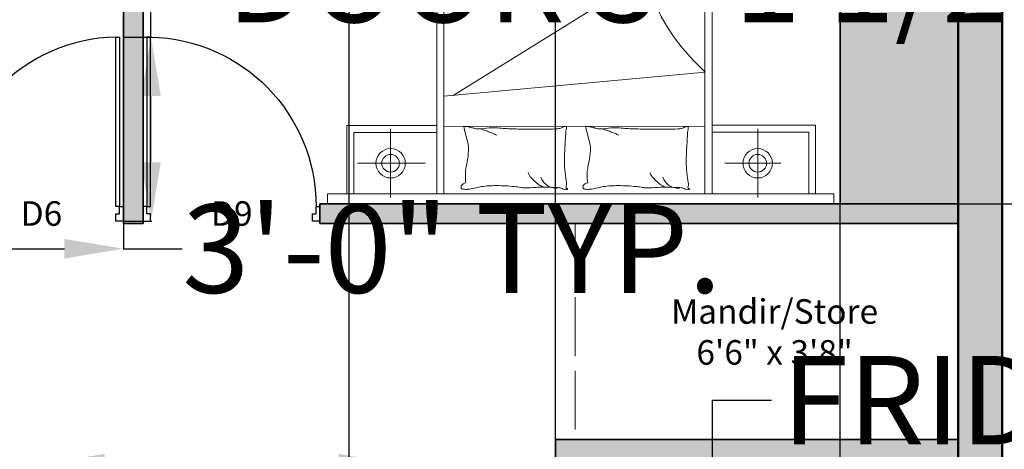
# Model space of a CAD drawing. Units: inches. Extents: x 2796 to 3603, y 978 to 1787.
# Tile 11 of 15: x 3224 to 3425, y 1458 to 1545. Entities that reach past the tile are written whole.
import ezdxf

# ---------------------------------------------------------------- set-up
doc = ezdxf.new("R2010")
doc.units = ezdxf.units.IN
doc.linetypes.add('ACAD_ISO02W100', pattern=[15, 12, -3])
for name, color, linetype, lineweight in [('A-ANNO-DIMS', 7, 'Continuous', 18), ('A-ANNO-TEXT', 7, 'Continuous', 18), ('A-AREA-IDEN', 7, 'Continuous', 18), ('A-DOOR', 6, 'Continuous', 25), ('A-FLOR-CASE', 2, 'Continuous', 25), ('A-FLOR-CASE-PATT', 2, 'Continuous', 13), ('A-FLOR-OVHD', 7, 'ACAD_ISO02W100', 18), ('A-WALL-EXTR-PATT', 1, 'Continuous', 13), ('A-WALL-INTR-PATT', 5, 'Continuous', 13), ('Furniture', 2, 'Continuous', 18), ('Inner Wall', 5, 'Continuous', 35), ('Outer Wall', 1, 'Continuous', 50)]:
    doc.layers.add(name, color=color, linetype=linetype, lineweight=lineweight)
doc.styles.get("Standard").update_dxf_attribs({"font": 'arial.ttf'})
doc.dimstyles.get("Standard").update_dxf_attribs({"dimtxt": 18, "dimasz": 12, "dimexe": 0.18, "dimexo": 0.0625, "dimgap": 0.09, "dimtad": 0, "dimtih": 1, "dimtoh": 1, "dimdec": 0, "dimzin": 0, "dimdsep": 46, "dimlunit": 3, "dimtxsty": 'Standard', "dimcen": 0.09, "dimadec": 0, "dimazin": 0, "dimtfac": 1, "dimtdec": 0, "dimtofl": 0, "dimtmove": 0, "dimatfit": 3, "dimfxl": 1, "dimtolj": 1, "dimtzin": 0, "dimarcsym": 0})

# ---------------------------------------------------------------- blocks, each defined once
blk = doc.blocks.new('A$C2B723114')
for p, q in [((0, 2.9047), (2.8274, 2.9047)), ((0, 2.8487), (0, 2.9047)), ((0.4243, 2.8697), (0.4243, 2.4855)), ((2.4742, 2.8697), (2.4742, 2.4855)), ((2.8274, 2.9047), (2.8274, 2.8487)), ((2.8274, 2.8487), (0, 2.8487)), ((0.1012, 2.4649), (0.1012, 2.849)), ((0.1396, 2.5033), (0.1396, 2.849)), ((0.6794, 0.7051), (0.6794, 2.8509)), ((0.7187, 0.7435), (0.7187, 2.8509)), ((2.1776, 2.8509), (2.1776, 0.7454)), ((2.216, 2.8509), (2.216, 0.707)), ((2.6798, 2.5052), (2.6798, 2.8509)), ((2.7182, 2.4668), (2.7182, 2.8509)), ((0.6087, 2.6776), (0.295, 2.6776)), ((2.6586, 2.6776), (2.2821, 2.6776)), ((1.3789, 2.4999), (1.3598, 2.5761)), ((2.0593, 2.4999), (2.0402, 2.5761)), ((0.6766, 2.5033), (0.1396, 2.5033)), ((1.3858, 2.4723), (1.3789, 2.4999)), ((2.0662, 2.4723), (2.0593, 2.4999)), ((2.2188, 2.5052), (2.6798, 2.5052)), ((0.6794, 2.4649), (0.1012, 2.4649)), ((0.7191, 2.47), (2.1778, 2.4719)), ((2.2188, 2.4668), (2.7182, 2.4668)), ((2.1771, 2.3036), (0.718, 2.1685)), ((1.0365, 1.6233), (2.1246, 2.2989)), ((2.2287, 1.6076), (2.2523, 1.5035)), ((0.5047, 1.5819), (0.5353, 1.4945)), ((0.6174, 1.5819), (0.6232, 1.4916)), ((0.6467, 1.5819), (0.6369, 1.5137)), ((0.6571, 1.4945), (0.6571, 1.5765)), ((2.2726, 1.593), (2.3061, 1.5007)), ((2.3067, 1.5881), (2.3373, 1.5007)), ((2.4194, 1.5881), (2.4251, 1.4979)), ((2.4487, 1.5881), (2.4389, 1.5199)), ((2.4591, 1.5007), (2.4591, 1.5828)), ((0.4269, 0.0884), (0.4269, 1.4945)), ((0.4269, 1.4945), (0.6794, 1.4945)), ((2.4685, 1.4964), (2.216, 1.5022)), ((2.4685, 1.4964), (2.4685, 0.0903)), ((0.3172, 1.3923), (0.4213, 1.3687)), ((2.4685, 1.4044), (2.5491, 1.3861)), ((0.3318, 1.3485), (0.4241, 1.3149)), ((2.4596, 1.3659), (2.552, 1.3324)), ((2.4645, 1.3318), (2.552, 1.3012)), ((0.3367, 1.3143), (0.4241, 1.2838)), ((2.4645, 1.2928), (2.5548, 1.2871)), ((2.4645, 1.2635), (2.5328, 1.2733)), ((2.4699, 1.2531), (2.552, 1.2163)), ((2.552, 1.2531), (2.4699, 1.2531)), ((2.5435, 1.2276), (2.4699, 1.2163)), ((2.4699, 1.2163), (2.5463, 1.1823)), ((0.3367, 1.2016), (0.427, 1.1959)), ((0.3367, 1.1724), (0.405, 1.1821)), ((0.4241, 1.162), (0.3421, 1.162)), ((0.3421, 1.162), (0.4241, 1.1252)), ((2.5491, 1.1654), (2.467, 1.1597)), ((2.5463, 1.1455), (2.467, 1.1342)), ((2.5491, 1.1342), (2.4699, 1.1201)), ((2.4699, 1.1201), (2.5491, 1.0946)), ((2.5463, 1.1172), (2.4727, 1.0918)), ((2.5491, 1.0946), (2.4699, 1.0635)), ((2.4699, 1.0635), (2.5491, 0.9842)), ((0.4157, 1.0206), (0.3421, 1.0093)), ((0.3421, 1.0093), (0.4185, 0.9754)), ((2.4642, 1.0267), (2.552, 0.9644)), ((0.4213, 0.9584), (0.3392, 0.9527)), ((0.4185, 0.9386), (0.3392, 0.9272)), ((2.4642, 0.9389), (2.4869, 0.9276)), ((2.467, 0.9559), (2.552, 0.9333)), ((2.4699, 0.9785), (2.552, 0.9531)), ((0.4213, 0.9272), (0.3421, 0.9131)), ((0.3421, 0.9131), (0.4213, 0.8876)), ((0.4213, 0.8876), (0.3421, 0.8565)), ((0.4185, 0.9103), (0.3449, 0.8848)), ((2.4642, 0.8908), (2.5152, 0.8483)), ((2.4869, 0.9276), (2.5265, 0.9163)), ((2.5265, 0.9163), (2.5491, 0.9163)), ((0.3421, 0.8565), (0.4213, 0.7772)), ((2.467, 0.8455), (2.5208, 0.8342)), ((2.5152, 0.8483), (2.5491, 0.837)), ((2.5208, 0.8342), (2.552, 0.8285)), ((2.552, 0.8285), (2.5293, 0.8087)), ((0.3364, 0.8197), (0.4241, 0.7574)), ((0.3421, 0.7716), (0.4241, 0.7461)), ((2.5491, 0.7606), (2.467, 0.7719)), ((2.4699, 0.8172), (2.4925, 0.7974)), ((2.5491, 0.8087), (2.4699, 0.8172)), ((2.4925, 0.7974), (2.535, 0.7889)), ((2.535, 0.7889), (2.552, 0.7861)), ((0.3392, 0.7489), (0.4241, 0.7263)), ((0.359, 0.7206), (0.3987, 0.7093)), ((2.1776, 0.7454), (0.7187, 0.7435)), ((2.4727, 0.7464), (2.467, 0.7408)), ((2.467, 0.7153), (2.5491, 0.7238)), ((2.552, 0.7464), (2.4727, 0.7464)), ((0.3421, 0.6601), (0.4213, 0.5808)), ((0.3987, 0.7093), (0.4213, 0.7093)), ((2.216, 0.707), (0.6794, 0.7051)), ((0.9938, 0.6115), (1.7555, 0.7064)), ((2.5491, 0.6842), (2.4642, 0.6615)), ((2.552, 0.7096), (2.467, 0.6842)), ((2.5491, 0.6672), (2.4755, 0.6587)), ((0.3364, 0.6233), (0.4241, 0.561)), ((2.4642, 0.6191), (2.4784, 0.6134)), ((2.4755, 0.6474), (2.5548, 0.6276)), ((2.4784, 0.6134), (2.5406, 0.6077)), ((2.5406, 0.6077), (2.552, 0.6134)), ((0.3392, 0.5525), (0.4241, 0.5299)), ((0.3421, 0.5752), (0.4241, 0.5497)), ((2.467, 0.5993), (2.4869, 0.5964)), ((2.467, 0.5313), (2.5491, 0.5596)), ((2.4869, 0.5964), (2.552, 0.5964)), ((0.359, 0.5242), (0.3987, 0.5129)), ((1.4523, 0.5021), (1.1305, 0.4537)), ((2.467, 0.5087), (2.5548, 0.5342)), ((2.5548, 0.5342), (2.4699, 0.4889)), ((0.3364, 0.4785), (0.3874, 0.436)), ((1.1305, 0.4537), (0.9938, 0.448)), ((0.4213, 0.415), (0.3364, 0.3923)), ((0.3392, 0.4332), (0.393, 0.4219)), ((0.4241, 0.2868), (0.3392, 0.415)), ((0.3421, 0.4049), (0.3647, 0.3851)), ((0.4213, 0.3964), (0.3421, 0.4049)), ((0.4213, 0.398), (0.3477, 0.3895)), ((0.3647, 0.3851), (0.4072, 0.3766)), ((0.3874, 0.436), (0.4213, 0.4247)), ((0.393, 0.4219), (0.4241, 0.4162)), ((0.4241, 0.4162), (0.4015, 0.3964)), ((2.467, 0.4133), (2.552, 0.4019)), ((2.467, 0.2879), (2.552, 0.4076)), ((0.4213, 0.3377), (0.3392, 0.3491)), ((0.4072, 0.3766), (0.4241, 0.3738)), ((0.3392, 0.2925), (0.4213, 0.3009)), ((0.4241, 0.3236), (0.3449, 0.3236)), ((2.4642, 0.3049), (2.5491, 0.2851)), ((2.467, 0.319), (2.5548, 0.3134)), ((0.3477, 0.2571), (0.427, 0.2373)), ((0.3506, 0.2231), (0.4128, 0.2175)), ((0.4128, 0.2175), (0.4241, 0.2231)), ((2.4699, 0.2491), (2.501, 0.2491)), ((2.501, 0.2491), (2.5491, 0.2547)), ((0.359, 0.2061), (0.4241, 0.2061)), ((2.467, 0.2179), (2.5605, 0.1981)), ((2.467, 0.1981), (2.5491, 0.1613)), ((2.467, 0.184), (2.4982, 0.1755)), ((2.4982, 0.1755), (2.5463, 0.1359)), ((0.3392, 0.1042), (0.4213, 0.1325)), ((2.4699, 0.1302), (2.535, 0.1104)), ((2.535, 0.1104), (2.5491, 0.0991)), ((0.3392, 0.0815), (0.427, 0.107)), ((0.427, 0.107), (0.3421, 0.0617)), ((2.4685, 0.0903), (0.4269, 0.0884)), ((0.5106, 0.0657), (0.5077, 0.0063)), ((0.5106, 0.094), (0.5106, 0.0657)), ((0.5417, 0.094), (0.5474, 0.0572)), ((0.5474, 0.0572), (0.57, 0.0006)), ((0.587, 0.0884), (0.604, 0.0346)), ((0.6512, 0.0884), (0.6682, 0.0346)), ((0.713, 0.0657), (0.7101, 0.0063)), ((0.713, 0.094), (0.713, 0.0657)), ((0.7334, 0.0943), (0.7503, 0.0434)), ((0.7786, 0.0915), (0.7786, 0.0632)), ((0.7786, 0.0632), (0.7843, 0.0066)), ((0.8739, 0.0884), (0.8908, 0.0346)), ((0.956, 0.0943), (0.973, 0.0434)), ((1.0013, 0.0915), (1.0013, 0.0632)), ((1.0013, 0.0632), (1.007, 0.0066)), ((1.072, 0.0884), (1.089, 0.0346)), ((1.1338, 0.0657), (1.131, 0.0063)), ((1.1338, 0.094), (1.1338, 0.0657)), ((1.1542, 0.0943), (1.1712, 0.0434)), ((1.1995, 0.0915), (1.1995, 0.0632)), ((1.1995, 0.0632), (1.2052, 0.0066)), ((1.4088, 0.0657), (1.406, 0.0063)), ((1.4088, 0.094), (1.4088, 0.0657)), ((1.44, 0.094), (1.4456, 0.0572)), ((1.4456, 0.0572), (1.4683, 0.0006)), ((1.4853, 0.0884), (1.5023, 0.0346)), ((1.5674, 0.0962), (1.5844, 0.0453)), ((1.6127, 0.0934), (1.6127, 0.0651)), ((1.6127, 0.0651), (1.6184, 0.0085)), ((1.6297, 0.0849), (1.624, 0.0028)), ((1.6693, 0.0623), (1.6608, 0.0028)), ((1.6721, 0.0877), (1.6693, 0.0623)), ((1.7344, 0.0651), (1.7316, 0.0057)), ((1.7344, 0.0934), (1.7344, 0.0651)), ((1.7655, 0.0934), (1.7712, 0.0566)), ((1.7712, 0.0566), (1.7938, 0)), ((1.8108, 0.0877), (1.8278, 0.034)), ((1.8568, 0.0962), (1.8738, 0.0453)), ((1.9342, 0.0962), (1.9512, 0.0453)), ((1.9795, 0.0934), (1.9795, 0.0651)), ((1.9795, 0.0651), (1.9852, 0.0085)), ((1.9965, 0.0849), (1.9908, 0.0028)), ((2.0361, 0.0623), (2.0276, 0.0028)), ((2.039, 0.0877), (2.0361, 0.0623)), ((2.1012, 0.0651), (2.0984, 0.0057)), ((2.1012, 0.0934), (2.1012, 0.0651)), ((2.1324, 0.0934), (2.138, 0.0566)), ((2.138, 0.0566), (2.1607, 0)), ((2.1777, 0.0877), (2.1946, 0.034)), ((2.2236, 0.0962), (2.2406, 0.0453)), ((2.2689, 0.0934), (2.2689, 0.0651)), ((2.2689, 0.0651), (2.2746, 0.0085)), ((2.2859, 0.0849), (2.2802, 0.0028)), ((2.3255, 0.0623), (2.317, 0.0028)), ((2.3284, 0.0877), (2.3255, 0.0623)), ((2.3906, 0.0651), (2.3878, 0.0057)), ((2.3906, 0.0934), (2.3906, 0.0651)), ((2.4218, 0.0934), (2.4274, 0.0566)), ((2.4274, 0.0566), (2.4501, 0)), ((2.4642, 0.0991), (2.5378, 0.0877)), ((2.467, 0.0877), (2.484, 0.034)), ((2.5378, 0.0877), (2.5463, 0.0821)), ((0.604, 0.0346), (0.621, 0.0063)), ((0.6682, 0.0346), (0.6851, 0.0063)), ((0.7503, 0.0434), (0.773, 0.0037)), ((0.8908, 0.0346), (0.9078, 0.0063)), ((0.973, 0.0434), (0.9957, 0.0037)), ((1.089, 0.0346), (1.106, 0.0063)), ((1.1712, 0.0434), (1.1939, 0.0037)), ((1.5023, 0.0346), (1.5192, 0.0082)), ((1.5844, 0.0453), (1.607, 0.0057)), ((1.8278, 0.034), (1.8448, 0.0057)), ((1.8738, 0.0453), (1.8964, 0.0057)), ((1.9512, 0.0453), (1.9739, 0.0057)), ((2.1946, 0.034), (2.2116, 0.0057)), ((2.2406, 0.0453), (2.2632, 0.0057)), ((2.484, 0.034), (2.501, 0.0057))]:
    blk.add_line(p, q)
for centre, radius in [((0.4243, 2.6776), 0.0821), ((2.4742, 2.6776), 0.0821), ((0.4243, 2.6776), 0.0493), ((2.4742, 2.6776), 0.0493)]:
    blk.add_circle(centre, radius)
for centre, radius, start, end in [((0.8078, 2.821), 0.00214, 160.436, 281.8931), ((0.8088, 2.8207), 0.00315, 111.7883, 160.436), ((0.8162, 2.8021), 0.0232, 94.3025, 111.7883), ((0.8091, 2.8151), 0.00394, 21.9904, 101.8931), ((0.8409, 2.7949), 0.0302, 158.579, 188.1335), ((0.7994, 2.8112), 0.0144, 338.579, 21.9904), ((0.8165, 2.7987), 0.0266, 59.3487, 94.3025), ((0.8554, 2.8643), 0.0497, 239.3487, 264.7408), ((0.9202, 3.5684), 0.7568, 264.7408, 268.0921), ((0.8679, 2.7254), 0.0915, 74.0648, 94.2159), ((0.8679, 2.7254), 0.0915, 53.9136, 74.0648), ((0.9409, 4.189), 1.3777, 268.0921, 270.5757), ((0.86, 2.6097), 0.2158, 62.7604, 69.1397), ((0.9466, 3.6164), 0.8051, 270.5757, 274.8018), ((1.0364, 2.548), 0.2671, 87.4614, 94.8018), ((1.042, 2.6745), 0.1405, 79.8101, 87.4614), ((1.1532, 3.2931), 0.488, 259.8101, 263.9133), ((1.204, 3.7695), 0.9671, 263.9133, 270), ((1.204, 3.4318), 0.6294, 270, 277.5469), ((1.2573, 3.0292), 0.2233, 277.5469, 285.744), ((1.3941, 2.5438), 0.281, 98.4372, 105.744), ((1.3747, 2.6748), 0.1486, 90, 98.4372), ((1.3713, 2.8186), 0.0315, 274.4002, 333.4195), ((1.3747, 2.74), 0.0833, 78.7276, 90), ((1.3886, 2.8099), 0.0121, 333.4195, 78.7276), ((1.4882, 2.821), 0.00214, 160.436, 281.8931), ((1.4892, 2.8207), 0.00315, 111.7883, 160.436), ((1.4966, 2.8021), 0.0232, 94.3025, 111.7883), ((1.4895, 2.8151), 0.00394, 21.9904, 101.8931), ((1.5213, 2.7949), 0.0302, 158.579, 188.1335), ((1.4798, 2.8112), 0.0144, 338.579, 21.9904), ((1.4969, 2.7987), 0.0266, 59.3487, 94.3025), ((1.5358, 2.8643), 0.0497, 239.3487, 264.7408), ((1.6006, 3.5684), 0.7568, 264.7408, 268.0921), ((1.5483, 2.7254), 0.0915, 74.0648, 94.2159), ((1.5483, 2.7254), 0.0915, 53.9136, 74.0648), ((1.6213, 4.189), 1.3777, 268.0921, 270.5757), ((1.5404, 2.6097), 0.2158, 62.7604, 69.1397), ((1.627, 3.6164), 0.8051, 270.5757, 274.8018), ((1.7168, 2.548), 0.2671, 87.4614, 94.8018), ((1.7224, 2.6745), 0.1405, 79.8101, 87.4614), ((1.8336, 3.2931), 0.488, 259.8101, 263.9133), ((1.8844, 3.7695), 0.9671, 263.9133, 270), ((1.8844, 3.4318), 0.6294, 270, 277.5469), ((1.9377, 3.0292), 0.2233, 277.5469, 285.744), ((2.0745, 2.5438), 0.281, 98.4372, 105.744), ((2.0551, 2.6748), 0.1486, 90, 98.4372), ((2.0517, 2.8186), 0.0315, 274.4002, 333.4195), ((2.0551, 2.74), 0.0833, 78.7276, 90), ((2.069, 2.8099), 0.0121, 333.4195, 78.7276), ((1.0356, 2.8227), 0.2268, 188.1335, 192.1095), ((0.635, 2.7368), 0.1829, 7.6809, 12.1095), ((-0.0181, 2.6487), 0.8418, 3.3687, 7.6809), ((0.8679, 2.7254), 0.0915, 36.1766, 53.9136), ((0.8679, 2.7254), 0.0915, 18.4397, 36.1766), ((0.9263, 2.7386), 0.0708, 51.6114, 62.7604), ((0.7461, 2.511), 0.3611, 46.1885, 51.6114), ((0.8523, 2.6218), 0.2076, 39.0349, 46.1885), ((0.9783, 2.7239), 0.0455, 28.3168, 39.0349), ((0.923, 2.7382), 0.4535, 0, 6.2324), ((1.716, 2.8227), 0.2268, 188.1335, 192.1095), ((1.3154, 2.7368), 0.1829, 7.6809, 12.1095), ((0.6623, 2.6487), 0.8418, 3.3687, 7.6809), ((1.5483, 2.7254), 0.0915, 36.1766, 53.9136), ((1.5483, 2.7254), 0.0915, 18.4397, 36.1766), ((1.6067, 2.7386), 0.0708, 51.6114, 62.7604), ((1.4265, 2.511), 0.3611, 46.1885, 51.6114), ((1.5327, 2.6218), 0.2076, 39.0349, 46.1885), ((1.6587, 2.7239), 0.0455, 28.3168, 39.0349), ((1.6034, 2.7382), 0.4535, 0, 6.2324), ((0.1976, 2.6614), 0.6258, 358.3669, 3.3687), ((0.8558, 2.6579), 0.1846, 23.0028, 28.3168), ((0.5722, 2.8434), 0.8132, 347.8016, 350.3156), ((1.1884, 2.7382), 0.1881, 350.3156, 0), ((0.878, 2.6614), 0.6258, 358.3669, 3.3687), ((1.5362, 2.6579), 0.1846, 23.0028, 28.3168), ((1.2526, 2.8434), 0.8132, 347.8016, 350.3156), ((1.8688, 2.7382), 0.1881, 350.3156, 0), ((-0.4351, 2.6794), 1.2587, 356.945, 358.3669), ((1.9648, 2.5659), 0.6074, 171.9949, 177.3351), ((1.6528, 2.6098), 0.2924, 167.8016, 171.9949), ((0.2453, 2.6794), 1.2587, 356.945, 358.3669), ((2.6452, 2.5659), 0.6074, 171.9949, 177.3351), ((2.3332, 2.6098), 0.2924, 167.8016, 171.9949), ((-11.7321, 3.2823), 12.5718, 356.49514, 356.94504), ((1.4204, 2.5912), 0.0624, 177.3351, 194.0452), ((-11.0517, 3.2823), 12.5718, 356.49514, 356.94504), ((2.1008, 2.5912), 0.0624, 177.3351, 194.0452), ((0.8298, 2.4774), 0.0178, 170.0016, 196.6978), ((0.5206, 2.5319), 0.2961, 350.0016, 356.4951), ((0.8068, 2.5419), 0.0707, 286.2212, 297.2841), ((0.8584, 2.4419), 0.0418, 102.869, 117.2841), ((0.879, 2.3515), 0.1345, 93.574, 102.869), ((0.9376, 1.4146), 1.0732, 90.2865, 93.574), ((0.9586, -2.7845), 5.2724, 89.0296, 90.2865), ((0.9954, -0.6123), 3.0999, 87.3904, 89.0296), ((1.0854, 1.364), 1.1216, 85.3824, 87.3904), ((1.28, 3.7729), 1.2952, 265.3824, 267.2509), ((1.4917, 3.1364), 0.681, 244.6889, 246.5156), ((1.228, 2.691), 0.2121, 267.2509, 281.5586), ((1.4917, 3.1364), 0.681, 246.5156, 248.3423), ((1.4917, 3.1364), 0.681, 248.3423, 250.572), ((1.4917, 3.1364), 0.681, 250.572, 252.8018), ((1.2975, 2.3514), 0.1345, 83.5659, 101.5586), ((1.3002, 2.3754), 0.1104, 72.6136, 83.5659), ((1.3965, 2.6828), 0.2118, 252.6136, 260.5159), ((1.5102, 2.4774), 0.0178, 170.0016, 196.6978), ((1.201, 2.5319), 0.2961, 350.0016, 356.4951), ((1.4872, 2.5419), 0.0707, 286.2212, 297.2841), ((1.5388, 2.4419), 0.0418, 102.869, 117.2841), ((1.5594, 2.3515), 0.1345, 93.574, 102.869), ((1.618, 1.4146), 1.0732, 90.2865, 93.574), ((1.639, -2.7845), 5.2724, 89.0296, 90.2865), ((1.6758, -0.6123), 3.0999, 87.3904, 89.0296), ((1.7658, 1.364), 1.1216, 85.3824, 87.3904), ((1.9604, 3.7729), 1.2952, 265.3824, 267.2509), ((2.1721, 3.1364), 0.681, 244.6889, 246.5156), ((1.9084, 2.691), 0.2121, 267.2509, 281.5586), ((2.1721, 3.1364), 0.681, 246.5156, 248.3423), ((2.1721, 3.1364), 0.681, 248.3423, 250.572), ((2.1721, 3.1364), 0.681, 250.572, 252.8018), ((1.9779, 2.3514), 0.1345, 83.5659, 101.5586), ((1.9806, 2.3754), 0.1104, 72.6136, 83.5659), ((2.0769, 2.6828), 0.2118, 252.6136, 260.5159), ((0.8139, 2.4726), 0.00122, 196.6978, 277.1204), ((0.8041, 2.5514), 0.0807, 277.1204, 286.2212), ((1.4027, 2.7202), 0.2496, 260.5159, 265.9171), ((1.385, 2.4721), 0.000845, 265.9171, 14.0449), ((1.4943, 2.4726), 0.00122, 196.6978, 277.1204), ((1.4845, 2.5514), 0.0807, 277.1204, 286.2212), ((2.0831, 2.7202), 0.2496, 260.5159, 265.9171), ((2.0654, 2.4721), 0.000845, 265.9171, 14.0449)]:
    blk.add_arc(centre, radius, start, end)
blk.add_ellipse((0.4962, 1.9132), major_axis=(0.4887, -0.4605), ratio=0.503305, start_param=0.491272, end_param=1.591113)
for points, knots in [([(0.6768, 1.3104), (0.6615, 1.3339), (0.6315, 1.3797), (0.604, 1.4501), (0.5417, 1.4748), (0.5064, 1.4871), (0.4848, 1.4945)], [0, 0, 0, 0, 110.980521, 216.571322, 273.316778, 363.252298, 363.252298, 363.252298, 363.252298]), ([(2.5548, 1.4853), (2.5314, 1.4757), (2.5031, 1.4641), (2.4737, 1.4555), (2.4685, 1.454)], [0, 0, 0, 0, 98.452083, 119.481049, 119.481049, 119.481049, 119.481049]), ([(0.427, 1.4678), (0.4036, 1.4582), (0.3693, 1.4441), (0.3335, 1.4344), (0.3221, 1.4313)], [0, 0, 0, 0, 98.452083, 144.639601, 144.639601, 144.639601, 144.639601]), ([(0.4241, 1.4423), (0.4031, 1.437), (0.3691, 1.4284), (0.3351, 1.4199), (0.3221, 1.4167)], [0, 0, 0, 0, 84.638756, 136.955563, 136.955563, 136.955563, 136.955563]), ([(2.552, 1.4598), (2.5309, 1.4545), (2.5031, 1.4475), (2.4753, 1.4406), (2.4685, 1.4389)], [0, 0, 0, 0, 84.638756, 111.94623, 111.94623, 111.94623, 111.94623]), ([(2.2145, 1.4211), (2.233, 1.4246), (2.2636, 1.4303), (2.2761, 1.3837), (2.3429, 1.3967), (2.3949, 1.3342), (2.4474, 1.3031), (2.4698, 1.2898)], [0, 0, 0, 0, 61.886907, 102.717887, 145.699352, 284.082577, 386.765171, 386.765171, 386.765171, 386.765171]), ([(0.6768, 1.286), (0.6567, 1.2911), (0.6145, 1.3017), (0.5543, 1.3533), (0.4816, 1.349), (0.4362, 1.3493), (0.4233, 1.3493)], [0, 0, 0, 0, 80.250278, 168.388677, 295.908361, 346.663112, 346.663112, 346.663112, 346.663112]), ([(0.4233, 1.3445), (0.4367, 1.3385), (0.464, 1.3264), (0.5129, 1.2848), (0.5456, 1.2161), (0.6131, 1.2349), (0.6142, 1.1913), (0.6642, 1.1806), (0.674, 1.144), (0.6817, 1.1154)], [0, 0, 0, 0, 56.745495, 115.23739, 254.956954, 286.678662, 337.828324, 366.201072, 468.500395, 468.500395, 468.500395, 468.500395]), ([(2.2145, 1.319), (2.2295, 1.319), (2.2678, 1.3192), (2.3288, 1.2705), (2.4143, 1.279), (2.4535, 1.2403), (2.4662, 1.2278)], [0, 0, 0, 0, 57.155505, 146.33427, 287.936209, 355.396728, 355.396728, 355.396728, 355.396728]), ([(2.3573, 1.127), (2.3656, 1.1759), (2.3758, 1.2352), (2.3371, 1.1853), (2.3602, 1.1713), (2.3768, 1.1612)], [0, 0, 0, 0, 107.853607, 130.728419, 189.220329, 189.220329, 189.220329, 189.220329]), ([(2.2182, 1.2059), (2.2419, 1.1958), (2.3116, 1.1659), (2.342, 1.0552), (2.4266, 1.0223), (2.4474, 0.9811), (2.462, 0.9684), (2.4698, 0.9616)], [0, 0, 0, 0, 97.73655, 287.59661, 389.176293, 423.403759, 463.679181, 463.679181, 463.679181, 463.679181]), ([(2.2145, 1.1476), (2.2246, 1.1286), (2.2575, 1.0666), (2.3612, 1.0009), (2.431, 0.9336), (2.4662, 0.8996)], [0, 0, 0, 0, 83.02987, 271.460712, 463.033803, 463.033803, 463.033803, 463.033803]), ([(0.6817, 0.8034), (0.6673, 0.8119), (0.6341, 0.8315), (0.5785, 0.8518), (0.5349, 0.8973), (0.4828, 0.9461), (0.4518, 0.9879), (0.4331, 1.013)], [0, 0, 0, 0, 65.318952, 150.437229, 226.833166, 307.58338, 429.454095, 429.454095, 429.454095, 429.454095]), ([(0.4282, 0.9448), (0.4547, 0.9353), (0.496, 0.9206), (0.5223, 0.8436), (0.5628, 0.7946), (0.6113, 0.7575), (0.6214, 0.7173), (0.6539, 0.7022), (0.672, 0.6897), (0.6768, 0.6864)], [0, 0, 0, 0, 102.299436, 159.044876, 303.717955, 348.579152, 391.138254, 454.581655, 477.456496, 477.456496, 477.456496, 477.456496]), ([(2.2145, 0.823), (2.227, 0.8201), (2.261, 0.8121), (2.261, 0.7401), (2.3352, 0.7659), (2.379, 0.6836), (2.4336, 0.6521), (2.4662, 0.6334)], [0, 0, 0, 0, 46.747668, 127.438174, 179.649794, 280.561838, 429.605131, 429.605131, 429.605131, 429.605131]), ([(0.4282, 0.74), (0.4347, 0.7029), (0.444, 0.6496), (0.5194, 0.6274), (0.555, 0.5807), (0.5975, 0.5243), (0.6789, 0.5415), (0.677, 0.5095), (0.6768, 0.5061)], [0, 0, 0, 0, 130.791737, 187.537266, 286.231946, 353.673191, 460.023761, 472.712403, 472.712403, 472.712403, 472.712403]), ([(2.2218, 0.7246), (2.2595, 0.716), (2.3548, 0.6945), (2.4265, 0.6268), (2.4698, 0.586)], [0, 0, 0, 0, 148.665024, 375.555892, 375.555892, 375.555892, 375.555892]), ([(2.3719, 0.6737), (2.3738, 0.6431), (2.3772, 0.5878), (2.3146, 0.6382), (2.3401, 0.7015), (2.2971, 0.6649), (2.2923, 0.6965), (2.289, 0.7176)], [0, 0, 0, 0, 83.446591, 150.887818, 201.642461, 230.015204, 286.760644, 286.760644, 286.760644, 286.760644]), ([(0.6768, 0.6864), (0.7275, 0.655), (0.8251, 0.5944), (0.9391, 0.606), (0.9938, 0.6115)], [0, 0, 0, 0, 225.995823, 434.686543, 434.686543, 434.686543, 434.686543]), ([(2.2145, 0.5167), (2.1764, 0.5522), (2.1051, 0.6184), (1.9357, 0.5803), (1.9385, 0.6342), (1.9388, 0.6395)], [0, 0, 0, 0, 208.073343, 389.01094, 409.01094, 409.01094, 409.01094, 409.01094]), ([(0.6768, 0.5061), (0.7554, 0.4794), (0.8591, 0.4442), (0.9675, 0.4473), (0.9938, 0.448)], [0, 0, 0, 0, 319.374611, 421.61723, 421.61723, 421.61723, 421.61723]), ([(0.4331, 0.4427), (0.4498, 0.4356), (0.4827, 0.4216), (0.5314, 0.3759), (0.632, 0.3884), (0.6996, 0.3513), (0.7423, 0.3278)], [0, 0, 0, 0, 70.931849, 139.556414, 248.154027, 434.709995, 434.709995, 434.709995, 434.709995]), ([(2.4625, 0.1088), (2.4095, 0.1438), (2.2904, 0.2226), (2.0623, 0.1771), (1.9006, 0.2246), (1.7699, 0.2337), (1.6941, 0.2766), (1.5528, 0.2786), (1.4005, 0.2587), (1.2324, 0.3267), (1.059, 0.2939), (0.9218, 0.426), (0.7359, 0.3204), (0.5586, 0.2391), (0.4502, 0.3116), (0.427, 0.3272)], [0, 0, 0, 0, 239.874704, 538.942419, 850.40885, 893.390315, 1047.998294, 1176.505142, 1437.500972, 1637.333004, 1864.324391, 2089.058767, 2248.736533, 2637.953392, 2744.252142, 2744.252142, 2744.252142, 2744.252142]), ([(1.9771, 0.0962), (1.9286, 0.1117), (1.7864, 0.157), (1.5223, 0.1992), (1.2611, 0.141), (1.0527, 0.2023), (0.8859, 0.1885), (0.76, 0.3042), (0.6211, 0.292), (0.5187, 0.3203), (0.4572, 0.3456), (0.4282, 0.3575)], [0, 0, 0, 0, 198.710624, 582.73994, 1031.873213, 1206.082894, 1423.278209, 1655.952104, 1808.744089, 1945.69963, 2068.229211, 2068.229211, 2068.229211, 2068.229211]), ([(0.8474, 0.0943), (0.82, 0.1047), (0.757, 0.1287), (0.6201, 0.1029), (0.4623, 0.1837), (0.4372, 0.2936), (0.4282, 0.3331)], [0, 0, 0, 0, 112.422038, 258.341957, 533.791494, 688.286079, 688.286079, 688.286079, 688.286079]), ([(0.8718, 0.2941), (0.8821, 0.3221), (0.9041, 0.3814), (0.9523, 0.2773), (0.8733, 0.2454), (0.8757, 0.2798), (0.8766, 0.2941)], [0, 0, 0, 0, 82.720021, 175.094899, 237.579423, 282.440623, 282.440623, 282.440623, 282.440623]), ([(1.2715, 0.221), (1.3344, 0.2172), (1.4529, 0.21), (1.2971, 0.2665), (1.2756, 0.2284), (1.2715, 0.221)], [0, 0, 0, 0, 150.888188, 283.977876, 315.699589, 315.699589, 315.699589, 315.699589])]:
    blk.add_open_spline(points, degree=3, knots=knots)
blk = doc.blocks.new('DOOR-SWING-36IN')
for points in [[(-0.01, 34.5), (-0.01, 0), (-0.76, 0), (-0.76, 34.5)], [(-35.26, -3), (-33.76, -3), (-33.76, -1.5), (-34.51, -1.5), (-34.51, 0), (-35.26, 0)], [(0.74, -3), (-0.76, -3), (-0.76, -1.5), (-0.01, -1.5), (-0.01, 0), (0.74, 0)]]:
    blk.add_lwpolyline(points, close=True)
blk.add_arc((0, 0), 34.51, 91.2592, 180)
blk = doc.blocks.new('*D18')
at = {"layer": 'A-ANNO-DIMS', "color": 0, "lineweight": -2, "transparency": 16777216}
for p, q in [((3250.87, 1541.68), (3250.87, 1553.68)), ((3250.87, 1553.68), (3262.87, 1553.68)), ((3245.31, 1541.68), (3251.05, 1541.68)), ((3250.87, 1516.18), (3250.87, 1529.68)), ((3245.31, 1504.18), (3251.05, 1504.18))]:
    blk.add_line(p, q, dxfattribs=at)
at = {"layer": 'A-ANNO-DIMS', "color": 0, "transparency": 16777216}
for points in [[(3248.87, 1529.68), (3252.87, 1529.68), (3250.87, 1541.68)], [(3248.87, 1516.18), (3252.87, 1516.18), (3250.87, 1504.18)]]:
    blk.add_solid(points, dxfattribs=at)
at = {"layer": 'Defpoints', "color": 0, "transparency": 16777216}
for p in [(3245.25, 1541.68), (3250.87, 1541.68), (3245.25, 1504.18)]:
    blk.add_point(p, dxfattribs=at)
at = {"layer": 'A-ANNO-DIMS', "color": 0, "transparency": 16777216, "insert": (3379.56, 1553.68), "char_height": 18, "attachment_point": 5}
blk.add_mtext('\\A1;DOOR 3\'-1 1/2" TYP.', dxfattribs=at)
blk = doc.blocks.new('*D19')
at = {"layer": 'A-ANNO-DIMS', "color": 0, "lineweight": -2, "transparency": 16777216}
for p, q in [((3209.25, 1504.11), (3209.25, 1498.37)), ((3245.25, 1504.11), (3245.25, 1498.37)), ((3221.25, 1498.55), (3233.25, 1498.55)), ((3245.25, 1498.55), (3257.25, 1498.55))]:
    blk.add_line(p, q, dxfattribs=at)
at = {"layer": 'A-ANNO-DIMS', "color": 0, "transparency": 16777216}
for points in [[(3221.25, 1500.55), (3221.25, 1496.55), (3209.25, 1498.55)], [(3233.25, 1500.55), (3233.25, 1496.55), (3245.25, 1498.55)]]:
    blk.add_solid(points, dxfattribs=at)
at = {"layer": 'Defpoints', "color": 0, "transparency": 16777216}
for p in [(3209.25, 1504.18), (3245.25, 1504.18), (3245.25, 1498.55)]:
    blk.add_point(p, dxfattribs=at)
at = {"layer": 'A-ANNO-DIMS', "color": 0, "transparency": 16777216, "insert": (3312.19, 1498.55), "char_height": 18, "attachment_point": 5}
blk.add_mtext('\\A1;3\'-0" TYP.', dxfattribs=at)
blk = doc.blocks.new('*D27')
at = {"layer": 'A-ANNO-DIMS', "color": 0, "lineweight": -2, "transparency": 16777216}
for p, q in [((3185.26, 1635.1), (3201.27, 1635.1)), ((3201.09, 1623.1), (3201.09, 1592.81)), ((3201.09, 1543.97), (3201.09, 1574.25)), ((3185.26, 1531.97), (3201.27, 1531.97))]:
    blk.add_line(p, q, dxfattribs=at)
at = {"layer": 'A-ANNO-DIMS', "color": 0, "transparency": 16777216}
for points in [[(3199.09, 1623.1), (3203.09, 1623.1), (3201.09, 1635.1)], [(3199.09, 1543.97), (3203.09, 1543.97), (3201.09, 1531.97)]]:
    blk.add_solid(points, dxfattribs=at)
at = {"layer": 'Defpoints', "color": 0, "transparency": 16777216}
for p in [(3185.2, 1635.1), (3201.09, 1635.1), (3185.2, 1531.97)]:
    blk.add_point(p, dxfattribs=at)
at = {"layer": 'A-ANNO-DIMS', "color": 0, "transparency": 16777216, "insert": (3201.09, 1583.53), "char_height": 18, "attachment_point": 5}
blk.add_mtext('\\A1;8\'-7" TYP.', dxfattribs=at)
blk = doc.blocks.new('*D32')
at = {"layer": 'A-ANNO-DIMS', "color": 0, "lineweight": -2, "transparency": 16777216}
for p, q in [((3229.46, 1454.75), (3217.46, 1454.75)), ((3229.46, 1444.07), (3229.46, 1454.93)), ((3289.09, 1454.75), (3241.46, 1454.75)), ((3301.09, 1444.07), (3301.09, 1454.93))]:
    blk.add_line(p, q, dxfattribs=at)
at = {"layer": 'A-ANNO-DIMS', "color": 0, "transparency": 16777216}
for points in [[(3241.46, 1456.75), (3241.46, 1452.75), (3229.46, 1454.75)], [(3289.09, 1456.75), (3289.09, 1452.75), (3301.09, 1454.75)]]:
    blk.add_solid(points, dxfattribs=at)
at = {"layer": 'Defpoints', "color": 0, "transparency": 16777216}
for p in [(3229.46, 1454.75), (3229.46, 1444.01), (3301.09, 1444.01)]:
    blk.add_point(p, dxfattribs=at)
at = {"layer": 'A-ANNO-DIMS', "color": 0, "transparency": 16777216, "insert": (3090.48, 1454.75), "char_height": 18, "attachment_point": 5}
blk.add_mtext('\\A1;DINING SET 5\'-11 1/2"', dxfattribs=at)
blk = doc.blocks.new('*D38')
at = {"layer": 'A-ANNO-DIMS', "color": 0, "lineweight": -2, "transparency": 16777216}
for p, q in [((3365.25, 1455.68), (3365.25, 1467.68)), ((3365.25, 1467.68), (3377.25, 1467.68)), ((3361.02, 1455.68), (3365.43, 1455.68)), ((3365.25, 1439.11), (3365.25, 1443.68)), ((3361.02, 1427.11), (3365.43, 1427.11))]:
    blk.add_line(p, q, dxfattribs=at)
at = {"layer": 'A-ANNO-DIMS', "color": 0, "transparency": 16777216}
for points in [[(3363.25, 1443.68), (3367.25, 1443.68), (3365.25, 1455.68)], [(3363.25, 1439.11), (3367.25, 1439.11), (3365.25, 1427.11)]]:
    blk.add_solid(points, dxfattribs=at)
at = {"layer": 'Defpoints', "color": 0, "transparency": 16777216}
for p in [(3360.96, 1455.68), (3365.25, 1455.68), (3360.96, 1427.11)]:
    blk.add_point(p, dxfattribs=at)
at = {"layer": 'A-ANNO-DIMS', "color": 0, "transparency": 16777216, "insert": (3472.71, 1467.68), "char_height": 18, "attachment_point": 5}
blk.add_mtext('\\A1;FRIDGE 2\'-4 1/2"', dxfattribs=at)
blk = doc.blocks.new('*D42')
at = {"layer": 'A-ANNO-DIMS', "color": 0, "lineweight": -2, "transparency": 16777216}
for p, q in [((3291.25, 1311.74), (3291.25, 1775.56)), ((3303.25, 1775.38), (3321.25, 1775.38)), ((3333.25, 1311.74), (3333.25, 1775.56)), ((3333.25, 1775.38), (3345.25, 1775.38))]:
    blk.add_line(p, q, dxfattribs=at)
at = {"layer": 'A-ANNO-DIMS', "color": 0, "transparency": 16777216}
for points in [[(3303.25, 1777.38), (3303.25, 1773.38), (3291.25, 1775.38)], [(3321.25, 1777.38), (3321.25, 1773.38), (3333.25, 1775.38)]]:
    blk.add_solid(points, dxfattribs=at)
at = {"layer": 'Defpoints', "color": 0, "transparency": 16777216}
for p in [(3333.25, 1775.38), (3291.25, 1311.68), (3333.25, 1311.68)]:
    blk.add_point(p, dxfattribs=at)
at = {"layer": 'A-ANNO-DIMS', "color": 0, "transparency": 16777216, "insert": (3369.25, 1775.38), "char_height": 18, "attachment_point": 5}
blk.add_mtext('\\A1;3\'-6"', dxfattribs=at)
blk = doc.blocks.new('*D49')
at = {"layer": 'A-ANNO-DIMS', "color": 0, "lineweight": -2, "transparency": 16777216}
for p, q in [((3415.31, 1603.68), (3463.13, 1603.68)), ((3462.95, 1591.68), (3462.95, 1564.96)), ((3462.95, 1519.68), (3462.95, 1546.4)), ((3415.31, 1507.68), (3463.13, 1507.68))]:
    blk.add_line(p, q, dxfattribs=at)
at = {"layer": 'A-ANNO-DIMS', "color": 0, "transparency": 16777216}
for points in [[(3460.95, 1591.68), (3464.95, 1591.68), (3462.95, 1603.68)], [(3460.95, 1519.68), (3464.95, 1519.68), (3462.95, 1507.68)]]:
    blk.add_solid(points, dxfattribs=at)
at = {"layer": 'Defpoints', "color": 0, "transparency": 16777216}
for p in [(3415.25, 1603.68), (3462.95, 1603.68), (3415.25, 1507.68)]:
    blk.add_point(p, dxfattribs=at)
at = {"layer": 'A-ANNO-DIMS', "color": 0, "transparency": 16777216, "insert": (3462.95, 1555.68), "char_height": 18, "attachment_point": 5}
blk.add_mtext('\\A1;8\'-0"', dxfattribs=at)
blk = doc.blocks.new('*D54')
at = {"layer": 'A-ANNO-DIMS', "color": 0, "lineweight": -2, "transparency": 16777216}
for p, q in [((3379.25, 1775.38), (3367.25, 1775.38)), ((3391.25, 1431.74), (3391.25, 1775.56)), ((3415.25, 1455.74), (3415.25, 1775.56)), ((3427.25, 1775.38), (3439.25, 1775.38))]:
    blk.add_line(p, q, dxfattribs=at)
at = {"layer": 'A-ANNO-DIMS', "color": 0, "transparency": 16777216}
for points in [[(3379.25, 1777.38), (3379.25, 1773.38), (3391.25, 1775.38)], [(3427.25, 1777.38), (3427.25, 1773.38), (3415.25, 1775.38)]]:
    blk.add_solid(points, dxfattribs=at)
at = {"layer": 'Defpoints', "color": 0, "transparency": 16777216}
for p in [(3415.25, 1775.38), (3415.25, 1455.68), (3391.25, 1431.68)]:
    blk.add_point(p, dxfattribs=at)
at = {"layer": 'A-ANNO-DIMS', "color": 0, "transparency": 16777216, "insert": (3463.41, 1775.38), "char_height": 18, "attachment_point": 5}
blk.add_mtext('\\A1;2\'-0"', dxfattribs=at)

msp = doc.modelspace()

# ---------------------------------------------------------------- hatches: boundary and pattern name
at = {"layer": 'A-FLOR-CASE-PATT'}
h = msp.add_hatch(dxfattribs=at)
h.set_pattern_fill('GOST_WOOD', color=256)
h.paths.add_polyline_path([(3127.25, 1727.68), (3079.25, 1727.68), (3079.25, 1703.68), (3127.25, 1703.68)])
h.paths.add_polyline_path([(3245.25, 1629.3), (3230.25, 1629.3), (3230.25, 1563.53), (3245.25, 1563.53)])
h.paths.add_polyline_path([(3381.25, 1651.68), (3315.48, 1651.68), (3315.48, 1636.68), (3381.25, 1636.68)])
h.paths.add_polyline_path([(3415.25, 1603.68), (3391.25, 1603.68), (3391.25, 1507.68), (3415.25, 1507.68)])
h.paths.add_polyline_path([(3199.25, 1407.44), (3184.25, 1407.44), (3184.25, 1353.68), (3199.25, 1353.68)])
h.paths.add_polyline_path([(3199.25, 1455.68), (3127.25, 1455.68), (3127.25, 1431.68), (3199.25, 1431.68)])
h.paths.add_polyline_path([(3223.25, 1244.56), (3208.25, 1244.56), (3208.25, 1178.79), (3223.25, 1178.79)])
h.paths.add_polyline_path([(3093.36, 1710.13), (3112.68, 1710.13), (3112.68, 1720.81), (3093.36, 1720.81)], flags=24)
h.paths.add_polyline_path([(3232.57, 1610.37), (3232.57, 1583.04), (3243.25, 1583.04), (3243.25, 1610.37)], flags=24)
h.paths.add_polyline_path([(3334.41, 1639), (3361.73, 1639), (3361.73, 1649.68), (3334.41, 1649.68)], flags=24)
h.paths.add_polyline_path([(3398.2, 1565.36), (3398.2, 1546.04), (3408.87, 1546.04), (3408.87, 1565.36)], flags=24)
h.paths.add_polyline_path([(3186.57, 1394.51), (3186.57, 1367.19), (3197.25, 1367.19), (3197.25, 1394.51)], flags=24)
h.paths.add_polyline_path([(3153.56, 1438.63), (3172.88, 1438.63), (3172.88, 1449.3), (3153.56, 1449.3)], flags=24)
h.paths.add_polyline_path([(3210.57, 1225.63), (3210.57, 1198.3), (3221.25, 1198.3), (3221.25, 1225.63)], flags=24)
at = {"layer": 'A-WALL-EXTR-PATT'}
h = msp.add_hatch(color=256, dxfattribs=at)
h.dxf.hatch_style = 1
h.paths.add_polyline_path([(3424.25, 1736.68), (3070.25, 1736.68), (3070.25, 1106.68), (3227.25, 1106.68), (3227.25, 1115.68), (3226.75, 1115.68), (3223.75, 1115.68), (3079.25, 1115.68), (3079.25, 1727.68), (3127.25, 1727.68), (3415.25, 1727.68), (3415.25, 1188.68), (3424.25, 1188.68)])
h.paths.add_polyline_path([(3291.25, 1032.68), (3074.25, 1032.68), (3074.25, 1106.68), (3070.25, 1106.68), (3070.25, 1028.68), (3291.25, 1028.68)])
h.paths.add_polyline_path([(3291.25, 1115.68), (3281.25, 1115.68), (3281.25, 1106.68), (3291.25, 1106.68)], flags=17)
h.paths.add_polyline_path([(3301.25, 1037.68), (3291.25, 1037.68), (3291.25, 1028.68), (3301.25, 1028.68)])
h.paths.add_polyline_path([(3424.25, 1037.68), (3414.25, 1037.68), (3414.25, 1028.68), (3424.25, 1028.68)])
h.paths.add_polyline_path([(3424.25, 1188.68), (3420.25, 1188.68), (3420.25, 1037.68), (3424.25, 1037.68)])
at = {"layer": 'A-WALL-INTR-PATT'}
h = msp.add_hatch(color=256, dxfattribs=at)
h.dxf.hatch_style = 1
h.paths.add_polyline_path([(3249.25, 1727.68), (3245.25, 1727.68), (3245.25, 1655.68), (3103.25, 1655.68), (3103.25, 1651.68), (3245.25, 1651.68), (3245.25, 1503.68), (3249.25, 1503.68)])
h.paths.add_polyline_path([(3131.25, 1727.68), (3127.25, 1727.68), (3127.25, 1703.68), (3127.25, 1679.68), (3131.25, 1679.68)], flags=17)
h.paths.add_polyline_path([(3391.25, 1655.68), (3325.25, 1655.68), (3325.25, 1727.68), (3321.25, 1727.68), (3321.25, 1655.68), (3273.25, 1655.68), (3273.25, 1651.68), (3391.25, 1651.68)])
h.paths.add_polyline_path([(3203.25, 1459.68), (3079.25, 1459.68), (3079.25, 1455.68), (3199.25, 1455.68), (3199.25, 1431.68), (3199.25, 1347.68), (3203.25, 1347.68)])
h.paths.add_polyline_path([(3209.25, 1507.68), (3079.25, 1507.68), (3079.25, 1503.68), (3209.25, 1503.68)])
h.paths.add_polyline_path([(3415.25, 1507.68), (3285.25, 1507.68), (3285.25, 1503.68), (3415.25, 1503.68)])
h.paths.add_polyline_path([(3415.25, 1459.68), (3333.25, 1459.68), (3333.25, 1455.68), (3415.25, 1455.68)])
h.paths.add_polyline_path([(3291.25, 1311.68), (3287.25, 1311.68), (3287.25, 1192.68), (3227.25, 1192.68), (3227.25, 1267.68), (3263.25, 1267.68), (3263.25, 1271.68), (3223.25, 1271.68), (3223.25, 1151.68), (3227.25, 1151.68), (3227.25, 1188.68), (3291.25, 1188.68)])
h.paths.add_polyline_path([(3227.25, 1311.68), (3079.25, 1311.68), (3079.25, 1307.68), (3227.25, 1307.68)])

# ---------------------------------------------------------------- linework, layer by layer
at = {"layer": 'A-FLOR-CASE'}
msp.add_lwpolyline([(3391.25, 1507.68), (3415.25, 1507.68), (3415.25, 1603.68), (3391.25, 1603.68)], close=True, dxfattribs=at)
at = {"layer": 'A-FLOR-OVHD'}
for p, q in [((3333.25, 1503.68), (3333.25, 1459.68)), ((3337.25, 1503.68), (3337.25, 1459.68))]:
    msp.add_line(p, q, dxfattribs=at)
at = {"layer": 'Inner Wall'}
for p, q in [((3249.25, 1503.68), (3249.25, 1727.68)), ((3245.25, 1503.68), (3245.25, 1651.68)), ((3415.25, 1507.68), (3285.25, 1507.68)), ((3285.25, 1503.68), (3285.25, 1507.68)), ((3245.25, 1503.68), (3249.25, 1503.68)), ((3285.25, 1503.68), (3415.25, 1503.68)), ((3333.25, 1459.68), (3415.25, 1459.68)), ((3333.25, 1455.68), (3333.25, 1459.68))]:
    msp.add_line(p, q, dxfattribs=at)
at = {"layer": 'Outer Wall'}
for p, q in [((3424.25, 1736.68), (3424.25, 1028.68)), ((3415.25, 1727.68), (3415.25, 1188.68))]:
    msp.add_line(p, q, dxfattribs=at)

# ---------------------------------------------------------------- block references
at = {"layer": 'A-DOOR'}
msp.add_blockref('DOOR-SWING-36IN', (3244.5, 1507.18), dxfattribs=at)
at = {"layer": 'A-DOOR', "extrusion": (0, 0, -1), "zscale": -1}
msp.add_blockref('DOOR-SWING-36IN', (-3249.99, 1507.18), dxfattribs=at)
at = {"layer": 'Furniture', "xscale": 36.47664764473289, "yscale": 36.47664764473289, "zscale": 36.47664764473289, "rotation": 180}
msp.add_blockref('A$C2B723114', (3389.93, 1613.63), dxfattribs=at)

# ---------------------------------------------------------------- texts
at = {"layer": 'A-ANNO-TEXT', "char_height": 5, "attachment_point": 3}
for s, insert in [('\\pxqc;{\\fTimes New Roman|b0|i0|c0|p18;D6}', (3236.4, 1508.22)), ('\\pxqc;{\\fTimes New Roman|b0|i0|c0|p18;D9}', (3275.16, 1508.22))]:
    msp.add_mtext_dynamic_manual_height_columns(s, width=15.6741, gutter_width=12.5, heights=[0], dxfattribs=dict(at, insert=insert))
at = {"layer": 'A-AREA-IDEN', "insert": (3405.64, 1488.26), "char_height": 5, "attachment_point": 3}
msp.add_mtext_dynamic_manual_height_columns('\\pxqc;{\\fTimes New Roman|b0|i0|c0|p18;Mandir/Store\\P6\'6" x 3\'8"}', width=55.5021, gutter_width=12.5, heights=[0], dxfattribs=at)

# ---------------------------------------------------------------- dimensions: what is measured, and where the dimension line sits
at = {"layer": 'A-ANNO-DIMS'}
for base, p1, p2, picture, middle in [((3333.25, 1775.38), (3291.25, 1311.68), (3333.25, 1311.68), '*D42', (3369.25, 1775.38)), ((3415.25, 1775.38), (3391.25, 1431.68), (3415.25, 1455.68), '*D54', (3463.41, 1775.38))]:
    dim = msp.add_linear_dim(base=base, p1=p1, p2=p2, dimstyle='Standard', override={"dimdec": 1, "dimlfac": 1, "dimrnd": 0, "dimzin": 1, "dimdsep": 46, "dimlunit": 4, "dimfrac": 2}, dxfattribs=at)
    dim.commit()
    dim.dimension.update_dxf_attribs({"geometry": picture, "text_midpoint": middle})
for base, p1, p2, angle, text, picture, middle in [((3201.09, 1635.1), (3185.2, 1531.97), (3185.2, 1635.1), 90, '<> TYP.', '*D27', (3201.09, 1583.53)), ((3250.87, 1541.68), (3245.25, 1504.18), (3245.25, 1541.68), 90, 'DOOR <> TYP.', '*D18', (3379.56, 1553.68)), ((3229.46, 1454.75), (3301.09, 1444.01), (3229.46, 1444.01), 180, 'DINING SET <>', '*D32', (3090.48, 1454.75)), ((3365.25, 1455.68), (3360.96, 1427.11), (3360.96, 1455.68), 90, 'FRIDGE <>', '*D38', (3472.71, 1467.68))]:
    dim = msp.add_linear_dim(base=base, p1=p1, p2=p2, angle=angle, text=text, dimstyle='Standard', override={"dimdec": 1, "dimlfac": 1, "dimrnd": 0, "dimzin": 1, "dimdsep": 46, "dimlunit": 4, "dimfrac": 2}, dxfattribs=at)
    dim.commit()
    dim.dimension.update_dxf_attribs({"geometry": picture, "text_midpoint": middle})
dim = msp.add_linear_dim(base=(3462.95, 1603.68), p1=(3415.25, 1507.68), p2=(3415.25, 1603.68), angle=90, dimstyle='Standard', override={"dimdec": 1, "dimlfac": 1, "dimrnd": 0, "dimzin": 1, "dimdsep": 46, "dimlunit": 4, "dimfrac": 2}, dxfattribs=at)
dim.commit()
dim.dimension.update_dxf_attribs({"geometry": '*D49', "text_midpoint": (3462.95, 1555.68)})
dim = msp.add_linear_dim(base=(3245.25, 1498.55), p1=(3209.25, 1504.18), p2=(3245.25, 1504.18), text='<> TYP.', dimstyle='Standard', override={"dimdec": 1, "dimlfac": 1, "dimrnd": 0, "dimzin": 1, "dimdsep": 46, "dimlunit": 4, "dimfrac": 2}, dxfattribs=at)
dim.commit()
dim.dimension.update_dxf_attribs({"geometry": '*D19', "text_midpoint": (3312.19, 1498.55)})

doc.saveas('drawing.dxf')
